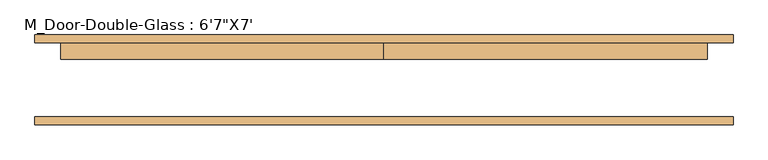
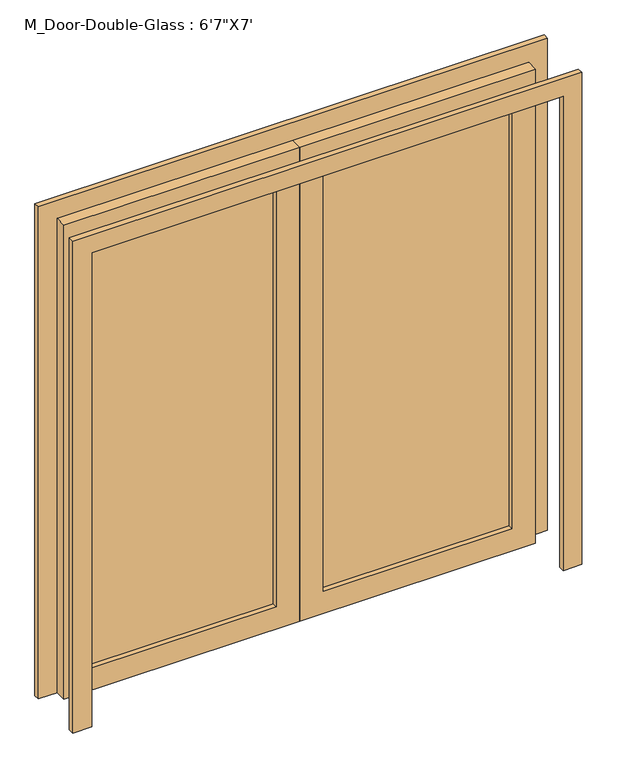
"""IFC4 building model written with IfcOpenShell, lengths in millimetres: door geometry."""

from ifc_helpers import new_model, si_unit, frame, origin, place, context, project, spatial, polyline, outline, extrude, source, transform, mapped, element, save


def door_77e2dd85(model_context):
    return source(origin(), model_context, "Body", "SweptSolid", [
        extrude(outline(polyline([(2133.6, 1003.3), (2133.6, 0.0), (0.0, 0.0), (0.0, 1003.3), (2133.6, 1003.3)]), holes=[polyline([(2033.6, 903.3), (100.0, 903.3), (100.0, 100.0), (2033.6, 100.0), (2033.6, 903.3)])]), frame((0.0, 66.68125, 0.0), z_axis=(0.0, 1.0, 0.0), x_axis=(0.0, 0.0, 1.0)), (0.0, 0.0, 1.0), 50.0),
        extrude(outline(polyline([(2133.6, -1003.3), (0.0, -1003.3), (0.0, 0.0), (2133.6, 0.0), (2133.6, -1003.3)]), holes=[polyline([(2033.6, -903.3), (2033.6, -100.0), (100.0, -100.0), (100.0, -903.3), (2033.6, -903.3)])]), frame((0.0, 66.68125, 0.0), z_axis=(0.0, 1.0, 0.0), x_axis=(0.0, 0.0, 1.0)), (0.0, 0.0, 1.0), 50.0),
        extrude(outline(polyline([(-903.3, 94.85625), (-100.0, 94.85625), (-100.0, 88.50625), (-903.3, 88.50625), (-903.3, 94.85625)])), frame((0.0, 0.0, 100.0), z_axis=(0.0, 0.0, 1.0), x_axis=(1.0, 0.0, 0.0)), (0.0, 0.0, 1.0), 1933.6),
        extrude(outline(polyline([(100.0, 94.85625), (903.3, 94.85625), (903.3, 88.50625), (100.0, 88.50625), (100.0, 94.85625)])), frame((0.0, 0.0, 100.0), z_axis=(0.0, 0.0, 1.0), x_axis=(1.0, 0.0, 0.0)), (0.0, 0.0, 1.0), 1933.6),
        extrude(outline(polyline([(0.0, 1083.3), (2213.6, 1083.3), (2213.6, -1083.3), (0.0, -1083.3), (0.0, -1003.3), (2133.6, -1003.3), (2133.6, 1003.3), (0.0, 1003.3), (0.0, 1083.3)])), frame((0.0, -136.91875, 0.0), z_axis=(0.0, 1.0, 0.0), x_axis=(0.0, 0.0, 1.0)), (0.0, 0.0, 1.0), 25.0),
        extrude(outline(polyline([(0.0, 1083.3), (2213.6, 1083.3), (2213.6, -1083.3), (0.0, -1083.3), (0.0, -1003.3), (2133.6, -1003.3), (2133.6, 1003.3), (0.0, 1003.3), (0.0, 1083.3)])), frame((0.0, 116.68125, 0.0), z_axis=(0.0, 1.0, 0.0), x_axis=(0.0, 0.0, 1.0)), (0.0, 0.0, 1.0), 25.0),
    ])


if __name__ == "__main__":
    model = new_model("IFC4")
    model_context = context("Model", 3, world=origin())
    ifc_project = project(units=[si_unit("LENGTHUNIT", "METRE", prefix="MILLI")], contexts=[model_context])
    site = spatial("IfcSite", under=ifc_project)
    building = spatial("IfcBuilding", under=site)
    placement = place(None, origin())
    door_shape = door_77e2dd85(model_context)
    element("IfcDoor", 1, ObjectType="M_Door-Double-Glass : 6'7\"X7'", at=placement, inside=building, context=model_context, shape_type="MappedRepresentation", body=[
        mapped(door_shape, transform((0.0, 0.0, 0.0), x_axis=(1.0, 0.0, 0.0), y_axis=(0.0, 1.0, 0.0), z_axis=(0.0, 0.0, 1.0))),
    ])
    save(model, "model.ifc")

# Revit data of these elements
# Type "M_Door-Double-Glass : 6'7\"X7'"
#   Type Mark = "16"
#   Construction Type Id = "opn-d45"
#   Assembly Code = "C1020"
#   Analytic Construction = "Wood frame, double glass door "
#   W = 3' - 3 1/2"
#   Thickness = 0' - 1.9685"
#   Thermal Resistance (R) = 1.8150 (h·ft²·°F)/BTU
#   Swing Angle [instance default] = 90.00°
#   Heat Transfer Coefficient (U) = 0.5510 BTU/(h·ft²·°F)
#   Height = 7' - 0"
#   Bottom Rail = 0' - 3.93701"
#   Top Rail = 0' - 3.93701"
#   Stiles = 0' - 3.93701"
#   Trim Projection = 0' - 0.98425"
#   Trim Width = 0' - 3.14961"
#   Width = 6' - 7"
#   Define Thermal Properties by = 1
#   Glazing = Glass
#   Panel Material = Wood - Birch - Solid Stained Light Low Gloss
#   Trim Material = Paint - Sienna
#   Visual Light Transmittance = 0
#   Solar Heat Gain Coefficient = 0
#   Function = (empty or 0)
#   Wall Closure = (empty or 0)
# Element 1 (IfcDoor, "M_Door-Double-Glass : 6'7\"X7'")
#   Materials on its faces: "Wood - Birch - Solid Stained Light Low Gloss", "Paint - Sienna", "Glass"
# Materials
#   "Glass": class "Glass", colour RGB 0 128 192, transparency 0.75, Description = "Soda Lime Glass", Cost = 0
#   "Wood - Birch - Solid Stained Light Low Gloss": class "Wood", colour RGB 210 159 95, transparency 0, Cost = 0
#   "Paint - Sienna": colour RGB 118 70 51, transparency 0, Cost = 0
